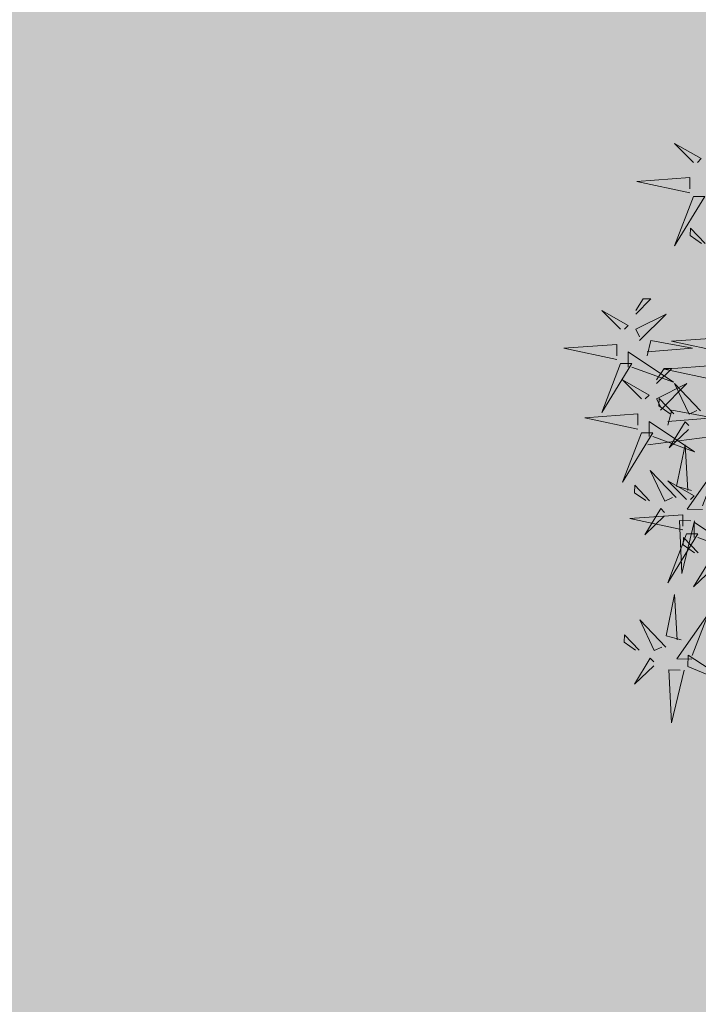
# Model space of a CAD drawing. Units: inches. Extents: x 1704 to 6393, y -157 to 1172.
# Tile 107 of 122: x 2667 to 2688, y 972 to 1003. Entities that reach past the tile are written whole.
import ezdxf

# ---------------------------------------------------------------- set-up
doc = ezdxf.new("R2010")
doc.units = ezdxf.units.IN
doc.header["$MEASUREMENT"] = 0
doc.layers.add('A-ANNO-DIMS', color=7, linetype='Continuous', lineweight=13)
doc.layers.add('L-shrub', color=74, linetype='Continuous', lineweight=18)
doc.layers.add('L-HRDS-PATT', color=9, linetype='Continuous', lineweight=13, true_color=0xc5c1ba)
doc.styles.get("Standard").update_dxf_attribs({"font": 'arial.ttf'})
doc.dimstyles.get("Standard").update_dxf_attribs({"dimtxt": 6, "dimasz": 2, "dimexe": 0.18, "dimexo": 0.0625, "dimgap": 0.09, "dimtad": 0, "dimtih": 1, "dimtoh": 1, "dimdec": 1, "dimzin": 0, "dimdsep": 46, "dimlunit": 3, "dimtxsty": 'Standard', "dimblk": 'ARCHTICK', "dimcen": 0.09, "dimadec": 0, "dimazin": 0, "dimtfac": 1, "dimtdec": 1, "dimtofl": 0, "dimtmove": 0, "dimatfit": 3, "dimfxl": 1, "dimtolj": 1, "dimtzin": 0, "dimarcsym": 0})

# ---------------------------------------------------------------- blocks, each defined once
blk = doc.blocks.new('shrub3')
blk.add_line((-16.77, -172.03), (-3.3, -276.98))
for points in [[(53.21, -248.82), (43.97, -248.82), (62.44, -221.15), (53.21, -246.52)], [(131.94, -252.6), (144.22, -222.89), (125.03, -252.43), (131.94, -252.6)], [(-59.53, -230.33), (-66.46, -262.61), (-68.77, -230.33), (-61.84, -230.33)], [(36.23, -243.83), (36, -253.06), (8.8, -233.9), (33.93, -243.77)], [(-42.57, -234.57), (-49.5, -266.85), (-51.81, -234.57), (-44.88, -234.57)], [(-15.2, -264.82), (-24.44, -262.51), (-19.82, -237.15), (-17.51, -264.82)], [(72.06, -237.38), (83.3, -249.21), (67.4, -239.57), (69.76, -237.32)], [(-175.52, -249.2), (-187.07, -260.73), (-177.83, -244.59), (-175.52, -246.89)], [(-154.74, -249.2), (-124.73, -260.73), (-154.74, -242.28), (-154.74, -249.2)], [(-126.07, -242.14), (-135.52, -251.14), (-130.91, -251.26), (-126.13, -244.45)], [(-24.09, -244.99), (-40.63, -260.74), (-21.96, -251.97), (-24.15, -247.3)], [(127.39, -250.18), (127.16, -259.41), (99.96, -240.26), (125.09, -250.12)], [(-157.05, -251.51), (-163.98, -283.79), (-166.29, -251.51), (-159.36, -251.51)], [(-57.6, -277.52), (-66.84, -275.22), (-62.22, -249.86), (-59.91, -277.52)], [(-8.28, -276.35), (-17.51, -276.35), (0.96, -248.68), (-8.28, -274.04)], [(-12.74, -252.2), (-1.5, -264.03), (-17.4, -254.39), (-15.04, -252.14)], [(24.53, -250.46), (22, -259.64), (-3.24, -254.39), (24.47, -252.77)], [(30.12, -253.43), (18.58, -264.96), (27.81, -248.82), (30.12, -251.13)], [(43.03, -248.62), (75.13, -256.35), (42.8, -257.85), (42.97, -250.92)], [(50.9, -253.43), (80.91, -264.96), (50.9, -246.52), (50.9, -253.43)], [(62.61, -246.38), (53.16, -255.38), (57.77, -255.49), (62.55, -248.69)], [(-24.44, -269.43), (-40.6, -253.29), (-31.36, -271.74), (-26.74, -269.43)], [(48.59, -255.74), (41.66, -288.02), (39.35, -255.74), (46.28, -255.74)], [(115.69, -256.81), (113.16, -265.99), (87.92, -260.74), (115.64, -259.12)], [(134.19, -254.97), (166.29, -262.7), (133.96, -264.2), (134.13, -257.28)], [(-50.68, -289.05), (-59.91, -289.05), (-41.44, -261.38), (-50.68, -286.75)], [(-40.6, -271.74), (-49.83, -262.51), (-49.83, -267.13), (-42.9, -271.74)], [(-22.19, -261.2), (-31.64, -270.2), (-27.03, -270.32), (-22.25, -263.51)], [(28.91, -259.81), (12.37, -275.56), (31.04, -266.79), (28.85, -262.12)], [(-66.84, -282.14), (-83, -266), (-73.76, -284.44), (-69.14, -282.14)], [(40.26, -267.02), (51.5, -278.85), (35.6, -269.21), (37.96, -266.96)], [(120.07, -266.16), (103.53, -281.91), (122.2, -273.14), (120.01, -268.47)], [(-83, -284.44), (-92.23, -275.22), (-92.23, -279.83), (-85.3, -284.44)], [(-10.58, -280.96), (19.43, -292.49), (-10.58, -274.04), (-10.58, -280.96)], [(30.81, -276.02), (21.36, -285.02), (25.97, -285.14), (30.75, -278.33)], [(131.42, -273.37), (142.66, -285.2), (126.76, -275.57), (129.12, -273.32)], [(-31.36, -280.96), (-42.9, -292.49), (-33.67, -276.35), (-31.36, -278.65)], [(-52.98, -293.67), (-22.97, -305.19), (-52.98, -286.75), (-52.98, -293.67)], [(-12.89, -283.27), (-19.82, -315.55), (-22.13, -283.27), (-15.2, -283.27)], [(121.97, -282.37), (112.52, -291.38), (117.13, -291.49), (121.91, -284.68)], [(-73.76, -293.67), (-85.3, -305.19), (-76.07, -289.05), (-73.76, -291.36)], [(-55.29, -295.97), (-62.22, -328.25), (-64.53, -295.97), (-57.6, -295.97)]]:
    blk.add_lwpolyline(points)
blk = doc.blocks.new('_ArchTick')
at = {"color": 0, "linetype": 'ByBlock', "const_width": 0.15}
blk.add_lwpolyline([(-0.5, -0.5), (0.5, 0.5)], dxfattribs=at)
blk = doc.blocks.new('*D95')
at = {"layer": 'A-ANNO-DIMS', "color": 0, "lineweight": -2, "transparency": 16777216}
for p, q in [((2605.349, 895.275), (2605.349, 1105.287)), ((2723.349, 895.275), (2723.349, 1105.287)), ((2605.349, 1105.107), (2657.907, 1105.107)), ((2723.349, 1105.107), (2670.791, 1105.107))]:
    blk.add_line(p, q, dxfattribs=at)
at = {"layer": 'Defpoints', "color": 0, "lineweight": -3, "transparency": 16777216}
for p in [(2723.349, 1105.107), (2605.349, 895.213), (2723.349, 895.213)]:
    blk.add_point(p, dxfattribs=at)
at = {"layer": 'A-ANNO-DIMS', "color": 0, "lineweight": -2, "transparency": 16777216, "xscale": 2, "yscale": 2, "zscale": 2, "rotation": 180}
blk.add_blockref('_ArchTick', (2605.349, 1105.107), dxfattribs=at)
at = {"layer": 'A-ANNO-DIMS', "color": 0, "lineweight": -2, "transparency": 16777216, "xscale": 2, "yscale": 2, "zscale": 2}
blk.add_blockref('_ArchTick', (2723.349, 1105.107), dxfattribs=at)
at = {"layer": 'A-ANNO-DIMS', "color": 0, "transparency": 16777216, "insert": (2664.349, 1105.107), "char_height": 6, "attachment_point": 5}
blk.add_mtext('\\A1;118', dxfattribs=at)

msp = doc.modelspace()

# ---------------------------------------------------------------- hatches: boundary and pattern name
at = {"layer": 'L-HRDS-PATT', "transparency": 33554661}
h = msp.add_hatch(color=256, dxfattribs=at)
h.dxf.hatch_style = 1
h.paths.add_polyline_path([(2719.349, 1033.213), (2664.349, 1033.213), (2664.349, 895.213), (2719.349, 895.213)])
h.paths.add_polyline_path([(2719.349, 895.213), (2664.349, 895.213), (2605.349, 895.213), (2605.349, 872.213), (2719.349, 872.213)])
h.paths.add_polyline_path([(2719.349, 872.213), (2605.349, 872.213), (2605.349, 854.213), (2601.349, 854.213, -0.121066), (2618.034, 850.113), (2618.05, 850.14), (2619.349, 849.39), (2601.349, 818.213), (2605.349, 818.213), (2605.349, 794.213), (2605.349, 754.213), (2631.349, 754.213), (2631.349, 716.213), (2719.349, 716.213)])

# ---------------------------------------------------------------- block references
at = {"layer": 'L-shrub', "xscale": 0.0510581485411622, "yscale": 0.0510581485411622, "zscale": 0.0510581485411622, "rotation": 269.9999999999999}
msp.add_blockref('shrub3', (2701.044, 989.25), dxfattribs=at)

# ---------------------------------------------------------------- dimensions: what is measured, and where the dimension line sits
at = {"layer": 'A-ANNO-DIMS'}
dim = msp.add_linear_dim(base=(2723.349, 1105.107), p1=(2605.349, 895.213), p2=(2723.349, 895.213), dimstyle='Standard', override={"dimdec": 0, "dimlfac": 1, "dimrnd": 0, "dimzin": 0, "dimdsep": 46, "dimlunit": 2}, dxfattribs=at)
dim.commit()
dim.dimension.update_dxf_attribs({"geometry": '*D95', "text_midpoint": (2664.349, 1105.107)})

doc.saveas('drawing.dxf')
